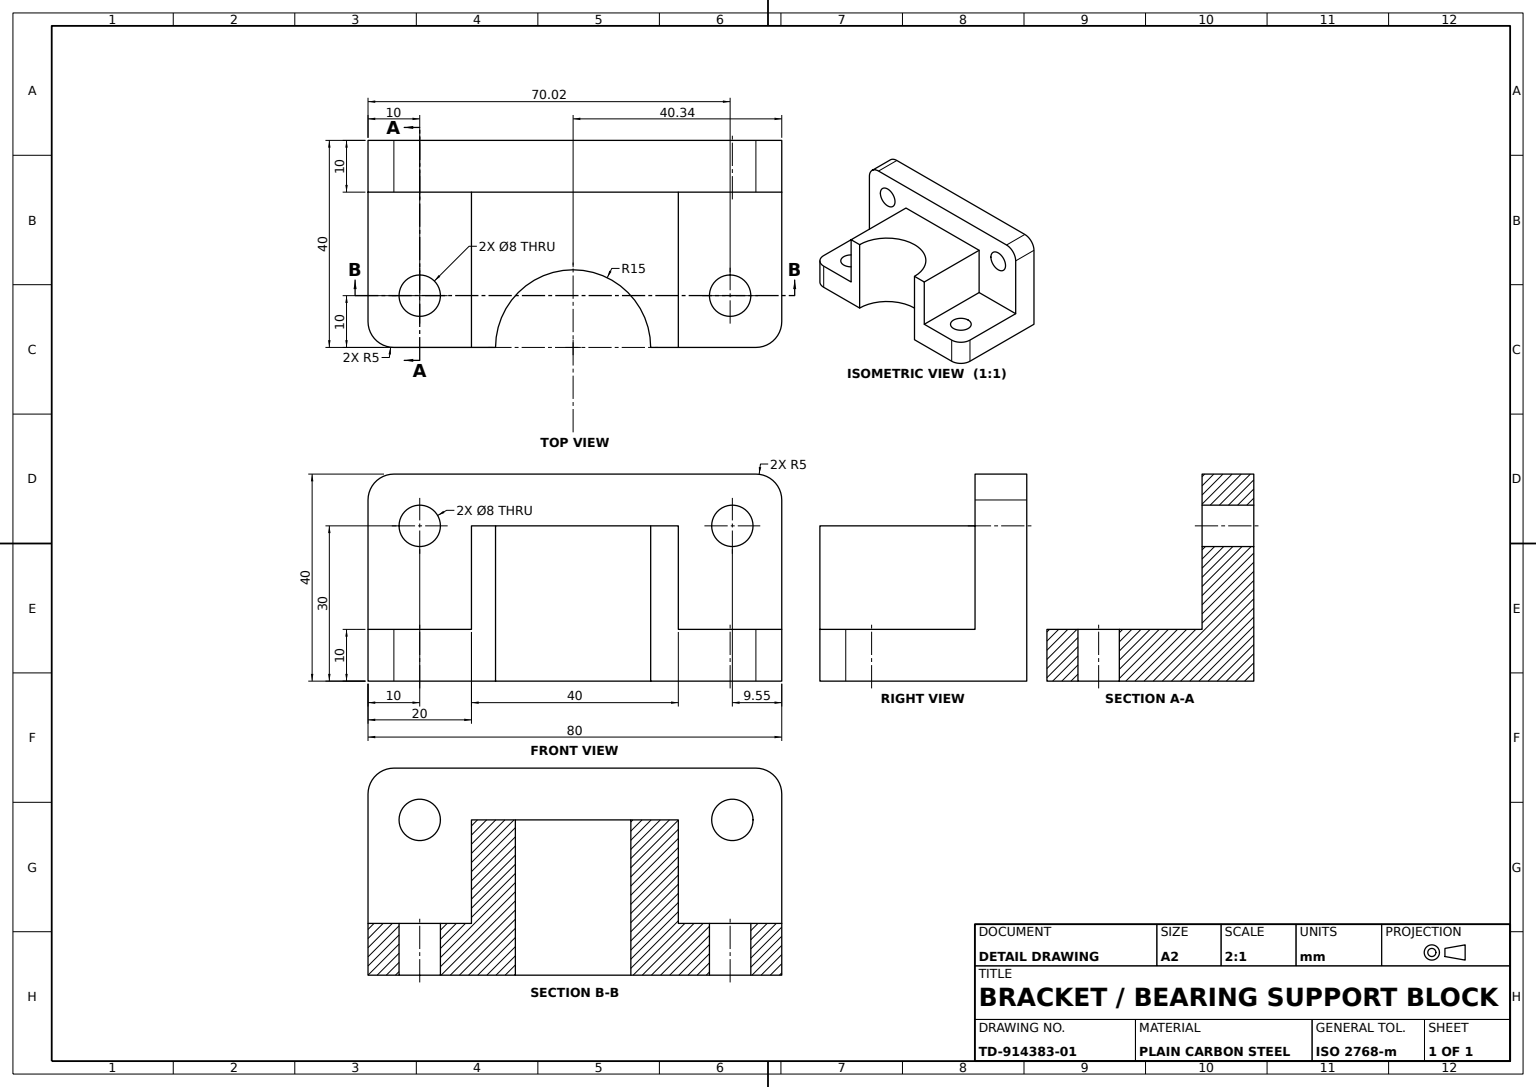
from build123d import *

# Parameters (mm, degrees)
BACK_PLATE_DEPTH            = 10
BASE_PLATE_DEPTH            = 10
BEARING_BLOCK_DEPTH         = 30
BACK_PLATE_HOLES_SKETCH_R   = 4
BACK_PLATE_HOLES_2X_8_DEPTH = 10
BASE_PLATE_HOLES_SKETCH_R   = 4
BASE_PLATE_HOLES_2X_8_DEPTH = 10


with BuildPart() as part:
    # Back Plate Sketch → Back Plate (new body)
    with BuildSketch(Plane.XY):
        with BuildLine():
            Line((0, 0), (80, 0))
            Line((80, 0), (80, 35))
            ThreePointArc((80, 35), (78.535533906, 38.535533906), (75, 40))
            Line((75, 40), (5, 40))
            ThreePointArc((5, 40), (1.464466094, 38.535533906), (0, 35))
            Line((0, 35), (0, 0))
        make_face()
    extrude(amount=BACK_PLATE_DEPTH)

    # Base Plate Sketch → Base Plate (add)
    with BuildSketch(Plane.XZ):
        with BuildLine():
            Line((0, 10), (0, 35))
            ThreePointArc((0, 35), (1.464466094, 38.535533906), (5, 40))
            Line((5, 40), (20, 40))
            Line((20, 40), (20, 10))
            Line((20, 10), (0, 10))
        make_face()
        with BuildLine():
            Line((80, 10), (80, 35))
            ThreePointArc((80, 35), (78.535533906, 38.535533906), (75, 40))
            Line((75, 40), (60, 40))
            Line((60, 40), (60, 10))
            Line((60, 10), (80, 10))
        make_face()
    extrude(amount=-BASE_PLATE_DEPTH)

    # Bearing Block Sketch → Bearing Block (add)
    with BuildSketch(Plane.XZ):
        with BuildLine():
            Line((20, 10), (20, 40))
            Line((20, 40), (24.655964266, 40))
            ThreePointArc((24.655964266, 40), (39.655964266, 25), (54.655964266, 40))
            Line((54.655964266, 40), (60, 40))
            Line((60, 40), (60, 10))
            Line((60, 10), (20, 10))
        make_face()
    extrude(amount=-BEARING_BLOCK_DEPTH)

    # Back Plate Holes Sketch → Back Plate Holes 2xØ8 (cut)
    with BuildSketch(Plane.XY.offset(10)):
        with Locations((10, 30)):
            Circle(BACK_PLATE_HOLES_SKETCH_R)
        with Locations((70.447162461, 30)):
            Circle(BACK_PLATE_HOLES_SKETCH_R)
    extrude(amount=-BACK_PLATE_HOLES_2X_8_DEPTH, mode=Mode.SUBTRACT)

    # Base Plate Holes Sketch → Base Plate Holes 2xØ8 (cut)
    with BuildSketch(Plane(origin=(0, 10, 0), x_dir=(1, 0, 0), z_dir=(0, 1, 0))):
        with Locations(Location((10, -30, 0), (0, 0, 270))):
            Circle(BASE_PLATE_HOLES_SKETCH_R)
        with Locations(Location((70.017117794, -30, 0), (0, 0, 270))):
            Circle(BASE_PLATE_HOLES_SKETCH_R)
    extrude(amount=-BASE_PLATE_HOLES_2X_8_DEPTH, mode=Mode.SUBTRACT)


solid = part.part
